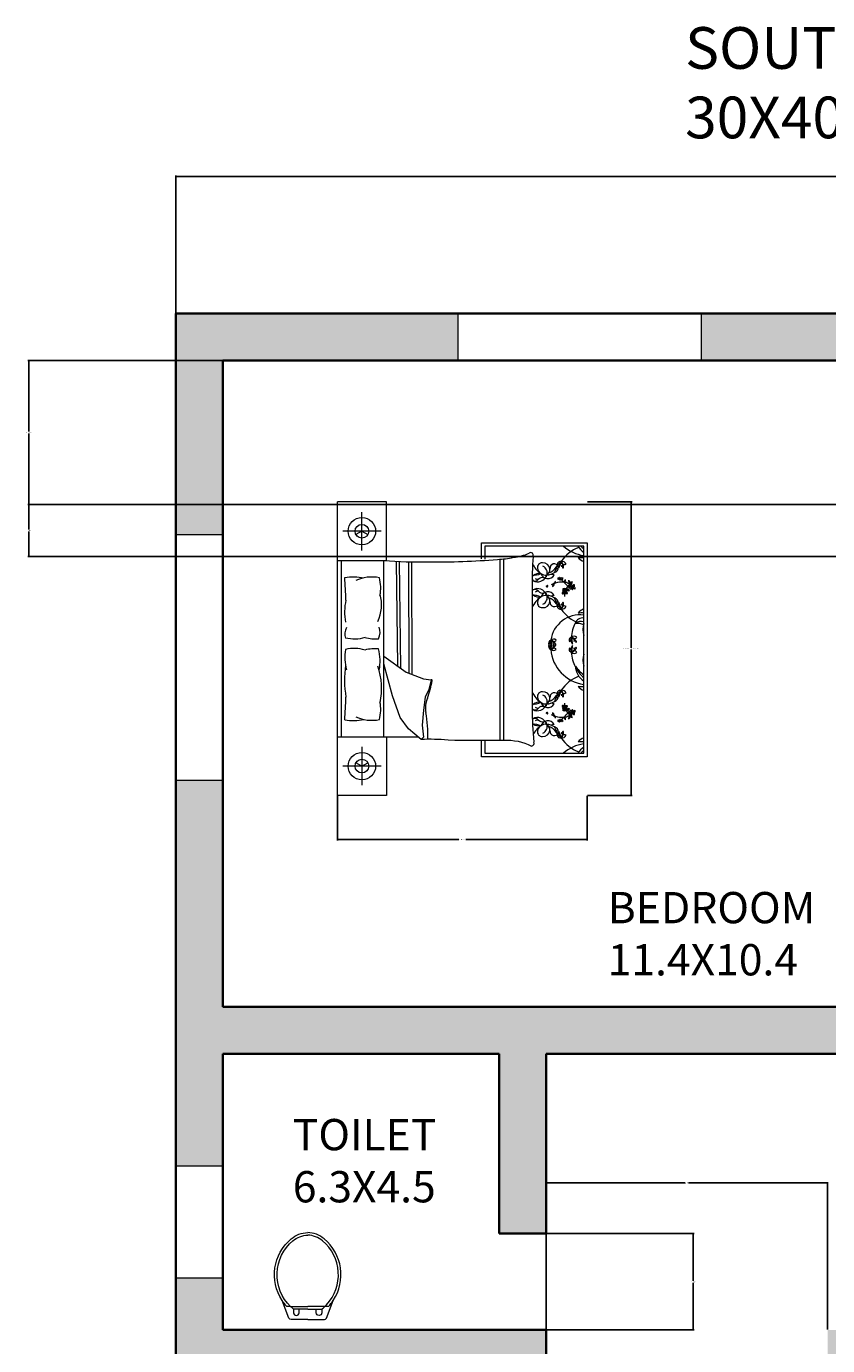
# Model space of a CAD drawing. Units: inches. Extents: x 8 to 486, y -516 to 97.
# Tile 3 of 5: x 8 to 162, y -185 to 68. Entities that reach past the tile are written whole.
import ezdxf

# ---------------------------------------------------------------- set-up
doc = ezdxf.new("R2010")
doc.units = ezdxf.units.IN
doc.header["$MEASUREMENT"] = 0
for name, color, linetype, lineweight in [('A-ANNO-DIMS', 2, 'Continuous', 18), ('A-ANNO-TEXT', 7, 'Continuous', 25), ('A-AREA-IDEN', 7, 'Continuous', 18), ('A-FLOR-FIXT', 9, 'Continuous', 18), ('A-FURN', 8, 'Continuous', 18), ('A-GLAZ', 4, 'Continuous', 18), ('A-WALL', 7, 'Continuous', 35), ('A-WALL-PATT', 150, 'Continuous', 13)]:
    doc.layers.add(name, color=color, linetype=linetype, lineweight=lineweight)
doc.styles.get("Standard").update_dxf_attribs({"font": 'arial.ttf'})
doc.dimstyles.get("Standard").update_dxf_attribs({"dimtxt": 0.18, "dimasz": 0.18, "dimexe": 0.18, "dimexo": 0.0625, "dimgap": 0.09, "dimtad": 0, "dimtih": 1, "dimtoh": 1, "dimdec": 0, "dimzin": 0, "dimdsep": 46, "dimlunit": 3, "dimtxsty": 'Standard', "dimcen": 0.09, "dimadec": 0, "dimazin": 0, "dimtfac": 1, "dimtdec": 0, "dimtofl": 0, "dimtmove": 0, "dimatfit": 3, "dimfxl": 1, "dimtolj": 1, "dimtzin": 0, "dimarcsym": 0})

# ---------------------------------------------------------------- blocks, each defined once
blk = doc.blocks.new('*D1')
at = {"layer": 'A-ANNO-DIMS', "color": 0, "lineweight": -2, "transparency": 16777216}
for p, q in [((37.13, 12.8), (37.13, 39.25)), ((37.31, 39.07), (214.23, 39.07)), ((411.95, 39.07), (235.02, 39.07)), ((412.13, 12.8), (412.13, 39.25))]:
    blk.add_line(p, q, dxfattribs=at)
at = {"layer": 'A-ANNO-DIMS', "color": 0, "transparency": 16777216}
for points in [[(37.31, 39.1), (37.31, 39.04), (37.13, 39.07)], [(411.95, 39.1), (411.95, 39.04), (412.13, 39.07)]]:
    blk.add_solid(points, dxfattribs=at)
at = {"layer": 'Defpoints', "color": 0, "transparency": 16777216}
for p in [(412.13, 39.07), (37.13, 12.74), (412.13, 12.74)]:
    blk.add_point(p, dxfattribs=at)
at = {"layer": 'A-ANNO-DIMS', "color": 0, "transparency": 16777216, "insert": (224.63, 39.07), "char_height": 6, "attachment_point": 5}
blk.add_mtext('\\A1;31\'-3"', dxfattribs=at)
blk = doc.blocks.new('BED-DOUBLE')
for p, q in [((0, 0), (0, 56.34)), ((4.7, 47.03), (4.7, 54.39)), ((8.38, 50.71), (1.01, 50.71)), ((27.62, 45.39), (27.62, 48.51)), ((27.62, 48.51), (47.92, 48.51)), ((47.92, 48.51), (47.92, 7.44)), ((28.27, 47.86), (28.27, 45.37)), ((47.26, 47.86), (28.27, 47.86)), ((47.26, 8.09), (47.26, 47.86)), ((0.72, 45.07), (0.72, 11.27)), ((8.9, 11.27), (8.9, 45.07)), ((11.24, 44.92), (11.53, 24.86)), ((11.82, 44.9), (12.11, 24.44)), ((13.6, 44.87), (13.68, 23.48)), ((14.18, 44.87), (14.26, 23.26)), ((31.13, 45.33), (31.13, 10.62)), ((31.84, 45.38), (31.84, 10.62)), ((41.55, 42.31), (40.91, 42.43)), ((37.37, 39.61), (37.37, 16.73)), ((41.55, 38.37), (40.91, 38.24)), ((8.9, 26.75), (13.2, 23.66)), ((10.58, 19.09), (8.9, 25.24)), ((13.2, 23.66), (16.51, 22.4)), ((16.51, 22.4), (17.99, 22.17)), ((17.54, 20.35), (16.85, 18.87)), ((17.99, 22.17), (17.54, 20.35)), ((12.06, 14.99), (10.58, 19.09)), ((16.85, 18.87), (16.51, 16.36)), ((16.51, 16.36), (16.28, 13.5)), ((41.55, 17.58), (40.91, 17.7)), ((13.66, 12.82), (12.06, 14.99)), ((16.05, 10.76), (13.66, 12.82)), ((16.28, 13.5), (16.51, 11.22)), ((41.55, 13.64), (40.91, 13.52)), ((0, 11.27), (15.46, 11.27)), ((16.51, 11.22), (16.05, 10.76)), ((27.62, 7.44), (27.62, 10.62)), ((28.27, 10.62), (28.27, 8.09)), ((4.7, 9.31), (4.7, 1.95)), ((28.27, 8.09), (47.26, 8.09)), ((8.38, 5.63), (1.01, 5.63)), ((47.92, 7.44), (27.62, 7.44))]:
    blk.add_line(p, q)
for points in [[(0, 45.07), (9.39, 45.07), (9.39, 56.34), (0, 56.34)], [(4.7, 50.71), (3.56, 50.05)], [(4.7, 50.71), (5.83, 50.05)], [(9.39, 11.27), (9.39, 0), (0, 0)], [(4.7, 5.63), (3.56, 6.29)], [(4.7, 5.63), (5.83, 6.29)]]:
    blk.add_lwpolyline(points)
for points in [[(30.69, 45.31, 0.056112), (33.79, 45.72, 0.095341), (36.78, 46.51)], [(1.4, 41.84, -0.074897), (5.08, 41.77, 0.472817)], [(5.29, 30.31, -0.14099), (1.54, 30.2, -0.235245)], [(5.29, 27.91, 0.14099), (1.54, 28.02, 0.235245)], [(1.4, 14.5, 0.074897), (5.08, 14.57, -0.472817)], [(21.21, 10.65, 0.001242), (31.9, 10.62, -0.127202), (37.23, 9.49)]]:
    blk.add_lwpolyline(points, format="xyb")
for centre, radius in [((4.7, 50.71), 2.63), ((4.7, 50.71), 1.31), ((43.59, 39.05), 0.143), ((45.1, 39.99), 0.143), ((43.59, 16.9), 0.143), ((45.1, 15.96), 0.143), ((4.7, 5.63), 2.63), ((4.7, 5.63), 1.31)]:
    blk.add_circle(centre, radius)
for centre, radius, start, end in [((37.06, 46.09), 0.514, 336.5219, 123.8264), ((92.17, 41.33), 54.82, 175.2402, 181.8035), ((48.98, 40.75), 7.36, 111.4092, 145.6135), ((48.25, 53.34), 7.36, 228.1144, 262.255), ((49.24, 49.64), 3.59, 209.8884, 236.5383), ((48.41, 47.64), 2.99, 221.0454, 247.4453), ((46.8, 55.83), 10.18, 266.3481, 272.5919), ((49.91, 50.93), 4.47, 223.5186, 233.6964), ((15.79, 146.07), 101.24, 266.1, 270.9282), ((19.47, 176.89), 132.06, 269.1145, 274.8735), ((41.34, 46.16), 4.26, 203.6453, 236.3329), ((39.29, 43.68), 0.951, 88.9462, 185.5144), ((39.99, 43.97), 1.69, 193.079, 274.7067), ((39.43, 43.29), 1.35, 7.1143, 95.0551), ((38.92, 42.76), 1.31, 338.5779, 68.4181), ((39.13, 43.52), 1.64, 305.9599, 357.6409), ((39.73, 45.27), 2.66, 288.2955, 328.7386), ((41.6, 43.6), 0.846, 19.1312, 189.736), ((41.34, 43.8), 1.06, 285.6955, 4.031), ((42.75, 42.66), 1.12, 128.4175, 173.8338), ((42.51, 43.77), 0.518, 126.7319, 206.0245), ((42.76, 44.31), 0.61, 76.272, 177.0484), ((41.84, 45.56), 1.26, 284.7031, 328.6173), ((43.59, 43.96), 1.16, 125.7657, 194.5347), ((37.88, 46.02), 5.15, 332.8176, 347.4827), ((43.08, 44.11), 0.816, 20.9613, 102.2885), ((43.52, 44.92), 0.614, 181.7131, 301.5367), ((41.51, 43.68), 1.86, 2.0648, 41.1598), ((42.63, 44.37), 0.602, 316.2238, 62.3173), ((42.98, 44.02), 0.048, 20.2667, 316.2271), ((43.23, 43.75), 0.0444, 52.0591, 168.5166), ((43.28, 43.74), 0.0914, 168.5166, 2.0648), ((-534.78, 10.78), 537.08, 2.8502, 3.3148), ((6.56, 34.66), 7.26, 78.2417, 114.8684), ((0.75, 39.83), 7.55, 348.9631, 14.8961), ((37.99, 41.7), 0.679, 196.6343, 225.5483), ((37.79, 44.6), 2.33, 259.249, 301.1782), ((37.99, 41.7), 0.679, 127.675, 162.5814), ((38.39, 42.79), 1.8, 240.8249, 340.7178), ((37.86, 41.99), 0.843, 246.1646, 318.4347), ((38.8, 40.44), 2.17, 85.2696, 124.215), ((38.72, 43.06), 1.62, 240.0851, 262.564), ((39.35, 40.67), 1.16, 74.8529, 138.4347), ((40.34, 43), 1.4, 196.8663, 330.0915), ((39.75, 42.12), 0.35, 254.8529, 12.6959), ((38.8, 40.44), 2.17, 53.6555, 57.2989), ((39.95, 45.3), 3.02, 273.4924, 303.7117), ((43.11, 36.27), 4.67, 110.1059, 116.9968), ((41.52, 40.48), 0.115, 83.9457, 185.6216), ((41.06, 40.58), 0.472, 328.836, 0.8141), ((41.3, 40.45), 0.27, 306.5232, 32.4668), ((41.62, 40.66), 0.115, 112.5583, 214.2343), ((41.55, 40.86), 0.27, 265.7131, 351.6568), ((41.31, 41.01), 0.472, 297.3659, 329.344), ((40.95, 41.42), 0.905, 313.6929, 321.7899), ((41.96, 40.8), 0.296, 115.5379, 168.6744), ((40.95, 41.22), 0.89, 329.344, 349.7412), ((43.11, 36.27), 4.67, 86.1723, 106.4158), ((40.24, 41.02), 1.59, 352.8698, 1.6736), ((42.35, 41.59), 0.111, 125.0752, 284.7644), ((42.52, 41.63), 0.239, 127.3642, 168.4363), ((42.33, 41.83), 0.345, 277.4968, 341.2737), ((42.6, 41.67), 0.137, 88.1325, 178.8919), ((42.88, 41.52), 0.297, 136.3462, 189.6513), ((42.71, 41.49), 0.124, 189.6513, 312.3208), ((42.74, 41.83), 0.143, 183.2768, 356.7232), ((43.19, 41.58), 0.47, 164.2829, 186.9148), ((42.63, 41.57), 0.235, 312.3208, 40.2111), ((43.13, 41.84), 0.333, 201.6382, 274.947), ((42.69, 41.38), 0.436, 42.3896, 66.5724), ((47.08, 44.83), 5.35, 217.9541, 226.8459), ((43, 41.64), 0.237, 10.9597, 52.2379), ((43.15, 41.62), 0.11, 274.947, 37.5263), ((43.52, 40.99), 0.115, 112.5583, 214.2343), ((43.45, 41.2), 0.27, 265.7131, 351.6568), ((43.21, 41.35), 0.472, 297.3659, 329.344), ((43.23, 38.6), 2.34, 60.7959, 85.244), ((38.25, 35.23), 7.7, 37.8256, 47.7588), ((42.85, 41.75), 0.905, 313.6929, 321.7899), ((43.85, 41.13), 0.296, 115.5379, 168.6744), ((42.85, 41.56), 0.89, 329.344, 349.7412), ((42.14, 41.35), 1.59, 352.8698, 1.6736), ((44.37, 41.03), 0.16, 33.0979, 123.1364), ((40.84, 38.77), 4.19, 31.1156, 34.8118), ((44.14, 40.76), 0.434, 2.3172, 70.5201), ((43.93, 40.29), 0.654, 310.9365, 22.7695), ((44.5, 40.65), 0.125, 135.7354, 318.1297), ((44.29, 40.86), 0.166, 315.7354, 31.1156), ((44.15, 40.5), 0.385, 319.3812, 5.5456), ((44.59, 40.65), 0.125, 68.2452, 250.6395), ((44.3, 40.81), 0.374, 352.6008, 57.1845), ((45.64, 38.3), 2.5, 111.7087, 116.2181), ((43.23, 38.6), 2.34, 47.5083, 55.9967), ((44.66, 40.89), 0.374, 252.8042, 349.6943), ((44.3, 40.22), 0.398, 331.1838, 51.6792), ((44.7, 40.92), 0.166, 248.2452, 323.6254), ((44.55, 41.02), 0.434, 291.7087, 3.0299), ((41.46, 43.31), 4.19, 323.6254, 327.3216), ((44.89, 40.92), 0.16, 325.6077, 55.6462), ((1.3, 36.57), 7.17, 333.8761, 16.1746), ((37.99, 38.97), 0.679, 134.4517, 156.7144), ((37.99, 38.97), 0.679, 203.2856, 232.325), ((37.79, 36.08), 2.33, 58.8218, 100.2867), ((41.34, 34.52), 4.26, 123.6671, 158.5059), ((38.39, 37.89), 1.8, 19.2822, 119.1751), ((37.86, 38.68), 0.843, 41.5653, 113.8354), ((38.8, 40.23), 2.17, 235.785, 274.7304), ((38.72, 37.62), 1.62, 97.436, 119.9149), ((39.99, 36.71), 1.69, 85.2933, 166.921), ((39.35, 40.01), 1.16, 221.5653, 285.1471), ((40.34, 37.67), 1.4, 29.9085, 163.1337), ((38.92, 37.92), 1.31, 291.5819, 21.4221), ((39.75, 38.56), 0.35, 347.3041, 105.1471), ((38.8, 40.23), 2.17, 302.7011, 306.3445), ((40.21, 40.19), 0.177, 169.5864, 349.5616), ((39.13, 37.16), 1.64, 2.3591, 54.0401), ((39.95, 35.38), 3.02, 56.2883, 86.5076), ((40.28, 40.18), 0.109, 349.5616, 167.2949), ((41.55, 40.12), 0.296, 129.5056, 182.6421), ((40.7, 40.8), 0.89, 308.4388, 328.836), ((40.54, 41.53), 1.59, 296.5064, 305.3102), ((40.53, 40.71), 0.905, 336.3901, 344.4871), ((43.2, 38.81), 0.111, 125.0752, 284.7644), ((43.37, 38.85), 0.239, 93.635, 168.4363), ((43.38, 40.15), 0.654, 253.6301, 325.4631), ((43.56, 39.24), 0.463, 82.0748, 142.6895), ((43.51, 39.88), 0.475, 228.342, 274.9894), ((43.34, 39.23), 0.141, 138.2946, 276.2474), ((43.39, 39.21), 0.196, 358.5719, 143.8954), ((43.18, 39.05), 0.345, 277.4968, 341.2737), ((43.46, 38.88), 0.137, 88.1325, 178.8919), ((43.51, 39.36), 0.197, 208.8493, 269.9355), ((43.34, 39.32), 0.226, 274.2123, 318.1587), ((43.73, 38.74), 0.297, 136.3462, 189.6513), ((43.56, 38.71), 0.124, 189.6513, 312.3208), ((46.34, 38.35), 2.81, 175.2415, 182.8929), ((43.52, 39.8), 0.398, 273.8774, 357.1501), ((44.04, 38.79), 0.47, 164.2829, 186.9148), ((44.03, 39.09), 0.452, 121.9501, 165.2442), ((43.68, 40.08), 0.385, 262.0748, 308.2393), ((43.49, 38.79), 0.235, 312.3208, 40.2111), ((43.98, 39.06), 0.333, 201.6382, 274.947), ((43.71, 39.26), 0.095, 262.868, 7.094), ((43.54, 38.6), 0.436, 42.3896, 66.5724), ((43.7, 39.34), 0.283, 278.5614, 22.5914), ((43.86, 38.86), 0.237, 10.9597, 118.7804), ((46.34, 38.35), 2.81, 156.1523, 156.9499), ((43.86, 39.35), 0.142, 44.3732, 121.9501), ((44.3, 39.69), 0.398, 181.4625, 249.4747), ((46.34, 38.35), 2.81, 130.182, 149.456), ((44.23, 40), 0.385, 215.1128, 261.2773), ((44.54, 39.98), 0.654, 197.889, 269.722), ((44, 38.83), 0.11, 274.947, 37.5263), ((44.34, 39.76), 0.475, 248.3627, 295.0101), ((44.1, 39.16), 0.463, 20.6625, 81.2773), ((44.79, 39.95), 0.463, 139.3812, 199.9959), ((44.23, 40.25), 0.475, 285.6484, 332.2957), ((44.71, 39.75), 0.111, 125.0752, 284.7644), ((44.88, 39.79), 0.239, 93.635, 168.4363), ((44.85, 40.17), 0.141, 138.2946, 276.2474), ((44.69, 39.98), 0.345, 277.4968, 341.2737), ((44.9, 40.15), 0.196, 358.5719, 143.8954), ((44.97, 39.82), 0.137, 88.1325, 178.8919), ((45.02, 40.3), 0.197, 208.8493, 269.9355), ((44.85, 40.26), 0.226, 274.2123, 318.1587), ((45.24, 39.68), 0.297, 136.3462, 189.6513), ((45.07, 39.65), 0.124, 189.6513, 312.3208), ((45.55, 39.73), 0.47, 164.2829, 186.9148), ((45.54, 40.03), 0.452, 121.9501, 165.2442), ((45, 39.73), 0.235, 312.3208, 40.2111), ((45.5, 39.99), 0.333, 201.6382, 274.947), ((45.23, 40.2), 0.095, 262.868, 7.094), ((45.05, 39.54), 0.436, 42.3896, 66.5724), ((45.21, 40.28), 0.283, 278.5614, 22.5914), ((45.37, 39.79), 0.237, 10.9597, 118.7804), ((45.37, 40.29), 0.142, 44.3732, 121.9501), ((45.52, 39.77), 0.11, 274.947, 37.5263), ((11.26, 35.15), 9.9, 166.3427, 191.1841), ((39.29, 37), 0.951, 174.4856, 271.0538), ((39.43, 37.39), 1.35, 264.9449, 352.8857), ((39.73, 35.4), 2.66, 31.2614, 71.7045), ((41.6, 37.08), 0.846, 170.264, 340.8688), ((42.75, 38.01), 1.12, 186.1662, 231.5825), ((41.34, 36.88), 1.06, 355.969, 74.3045), ((42.51, 36.91), 0.518, 153.9755, 233.2681), ((42.76, 36.36), 0.61, 182.9516, 283.728), ((41.84, 35.12), 1.26, 31.3827, 75.2969), ((43.59, 36.72), 1.16, 165.4653, 234.2343), ((37.88, 34.66), 5.15, 12.5173, 27.1824), ((41.51, 37), 1.86, 318.8402, 357.9352), ((42.63, 36.3), 0.602, 297.6827, 43.7762), ((43.52, 35.75), 0.614, 58.4633, 178.2869), ((43.08, 36.57), 0.816, 257.7115, 339.0387), ((48.98, 39.93), 7.36, 214.3865, 248.5908), ((43.01, 36.67), 0.0796, 43.7762, 339.7183), ((43.28, 36.93), 0.0914, 357.9352, 191.4834), ((43.23, 36.92), 0.0444, 191.4834, 307.9409), ((48.41, 33.04), 2.99, 112.5547, 138.9546), ((46.55, 28.98), 5.69, 82.8636, 171.8197), ((52.19, 29.78), 7.36, 152.5854, 175.5377), ((46.95, 32.74), 1.32, 76.3898, 169.0739), ((46.77, 31.74), 1.67, 72.8609, 131.9049), ((46.03, 29.72), 3.29, 68.117, 96.6195), ((46.8, 24.84), 10.18, 87.4081, 93.6519), ((51.13, 31.84), 4.05, 162.9798, 196.4569), ((4.21, 30.97), 2.79, 153.3437, 196.1026), ((5.19, 31.35), 2.99, 335.0183, 18.5407), ((45.41, 29.75), 0.816, 50.8855, 132.2127), ((45.38, 30.68), 0.614, 211.6373, 331.4609), ((53.22, 30.24), 5.98, 174.3643, 175.6213), ((57.31, 27.08), 10.69, 160.0972, 160.2783), ((11.47, 26.54), 10.04, 171.5249, 193.96), ((7.17, 36.95), 6.9, 254.1707, 275.9871), ((7.17, 21.26), 6.9, 84.0129, 105.8293), ((-1.76, 25.79), 9.94, 349.8617, 13.6238), ((41.09, 29.2), 0.61, 106.1963, 206.9726), ((41.09, 28.62), 0.61, 153.0274, 253.8037), ((39.66, 29.82), 1.26, 314.6273, 358.5415), ((39.66, 28), 1.26, 1.4585, 45.3727), ((41.98, 29.31), 1.16, 155.6899, 224.4589), ((41.98, 28.51), 1.16, 135.5411, 204.3101), ((41.47, 29.19), 0.816, 50.8855, 132.2127), ((41.44, 30.11), 0.614, 211.6373, 331.4609), ((40.94, 29.19), 0.602, 346.148, 92.2415), ((40.32, 28.03), 1.86, 31.989, 71.0841), ((36.01, 28.25), 5.15, 2.7418, 17.407), ((36.01, 29.58), 5.15, 342.593, 357.2582), ((40.32, 29.8), 1.86, 288.9159, 328.011), ((40.94, 28.64), 0.602, 267.7585, 13.852), ((41.44, 27.71), 0.614, 28.5391, 148.3627), ((41.47, 28.64), 0.816, 227.7873, 309.1145), ((48.25, 28.61), 7.36, 184.4623, 262.255), ((41.42, 29.06), 0.048, 50.1909, 346.0209), ((41.45, 28.76), 0.0796, 13.852, 309.9245), ((41.82, 28.97), 0.0914, 198.4408, 31.989), ((41.77, 28.95), 0.0444, 81.9833, 198.4408), ((41.82, 28.86), 0.0914, 328.011, 161.5592), ((41.77, 28.87), 0.0444, 161.5592, 278.0167), ((45.03, 29.77), 0.61, 106.1963, 206.9726), ((45.03, 28.06), 0.61, 153.0274, 253.8037), ((43.6, 30.38), 1.26, 314.6273, 358.5415), ((43.6, 27.44), 1.26, 1.4585, 45.3727), ((45.92, 29.87), 1.16, 155.6899, 224.4589), ((45.92, 27.95), 1.16, 135.5411, 204.3101), ((44.26, 28.59), 1.86, 31.989, 71.0841), ((39.95, 28.81), 5.15, 2.7418, 17.407), ((44.88, 29.75), 0.602, 346.148, 92.2415), ((39.95, 29.01), 5.15, 342.593, 357.2582), ((44.26, 29.23), 1.86, 288.9159, 328.011), ((44.88, 28.07), 0.602, 267.7585, 13.852), ((45.36, 29.62), 0.048, 50.1909, 346.0209), ((45.39, 28.2), 0.0796, 13.852, 309.9245), ((45.76, 29.53), 0.0914, 198.4408, 31.989), ((45.71, 29.52), 0.0444, 81.9833, 198.4408), ((45.76, 28.3), 0.0914, 328.011, 161.5592), ((45.71, 28.31), 0.0444, 161.5592, 278.0167), ((45.38, 27.15), 0.614, 28.5391, 148.3627), ((45.41, 28.08), 0.816, 227.7873, 309.1145), ((52.19, 28.04), 7.36, 184.4623, 207.4146), ((51.13, 25.99), 4.05, 163.5431, 197.0202), ((53.22, 27.59), 5.98, 184.3787, 185.6357), ((57.31, 30.74), 10.69, 199.7217, 199.9028), ((21.79, 22.22), 20.43, 172.2196, 189.497), ((-4.62, 20.49), 13.1, 348.0397, 19.2615), ((48.98, 16.02), 7.36, 111.4092, 145.6135), ((49.24, 24.92), 3.59, 181.272, 236.5383), ((51.16, 28.56), 6.65, 214.0123, 234.053), ((49.91, 26.21), 4.47, 197.8504, 233.6964), ((-3.3, 26.09), 21.85, 340.1194, 349.3383), ((18.04, 22.05), 0.136, 358.8623, 109.7536), ((46.8, 31.1), 10.18, 266.3481, 272.5919), ((48.41, 22.91), 2.99, 221.0454, 247.4453), ((-534.78, 45.56), 537.08, 356.6852, 357.1498), ((0.75, 16.51), 7.55, 345.1039, 11.0369), ((21.45, 16.81), 4.59, 156.2616, 191.3392), ((41.34, 21.43), 4.26, 201.4941, 236.3329), ((37.79, 19.87), 2.33, 259.7133, 301.1782), ((38.8, 15.72), 2.17, 85.2696, 124.215), ((39.29, 18.95), 0.951, 88.9462, 185.5144), ((39.99, 19.24), 1.69, 193.079, 274.7067), ((40.34, 18.28), 1.4, 196.8663, 330.0915), ((39.43, 18.56), 1.35, 7.1143, 95.0551), ((38.92, 18.03), 1.31, 338.5779, 68.4181), ((39.13, 18.79), 1.64, 305.9599, 357.6409), ((39.95, 20.57), 3.02, 273.4924, 303.7117), ((39.73, 20.54), 2.66, 288.2955, 328.7386), ((41.6, 18.87), 0.846, 19.1312, 189.736), ((41.34, 19.07), 1.06, 285.6955, 4.031), ((42.75, 17.93), 1.12, 128.4175, 173.8338), ((42.51, 19.04), 0.518, 126.7319, 206.0245), ((42.76, 19.58), 0.61, 76.272, 177.0484), ((41.84, 20.83), 1.26, 284.7031, 328.6173), ((43.59, 19.23), 1.16, 125.7657, 194.5347), ((37.88, 21.29), 5.15, 332.8176, 347.4827), ((43.08, 19.38), 0.816, 20.9613, 102.2885), ((42.63, 19.64), 0.602, 316.2238, 62.3173), ((41.51, 18.95), 1.86, 2.0648, 41.1598), ((43.52, 20.19), 0.614, 181.7131, 301.5367), ((42.98, 19.29), 0.048, 20.2667, 316.2271), ((43.23, 19.02), 0.0444, 52.0591, 168.5166), ((43.28, 19.02), 0.0914, 168.5166, 2.0648), ((46.34, 17.59), 2.81, 177.1071, 184.7585), ((-3.9, 11.73), 21.26, 357.4519, 11.3392), ((37.99, 16.98), 0.679, 127.675, 156.7144), ((96.02, 16.06), 58.65, 179.3433, 185.6887), ((37.99, 16.98), 0.679, 203.229, 225.5483), ((38.39, 18.06), 1.8, 240.8249, 340.7178), ((37.86, 17.26), 0.843, 246.1646, 318.4347), ((38.72, 18.33), 1.62, 240.0851, 262.564), ((39.35, 15.94), 1.16, 74.8529, 138.4347), ((39.75, 17.39), 0.35, 254.8529, 12.6959), ((38.8, 15.72), 2.17, 53.6555, 57.2989), ((40.21, 15.76), 0.177, 10.4384, 190.4136), ((40.28, 15.77), 0.109, 192.7051, 10.4384), ((43.11, 19.68), 4.67, 243.0032, 249.8941), ((40.7, 15.15), 0.89, 31.164, 51.5612), ((41.55, 15.83), 0.296, 177.3579, 230.4944), ((40.54, 14.42), 1.59, 54.6898, 63.4936), ((40.53, 15.24), 0.905, 15.5129, 23.6099), ((41.52, 15.47), 0.115, 174.3784, 276.0543), ((41.3, 15.5), 0.27, 327.5332, 53.4768), ((41.06, 15.36), 0.472, 359.1859, 31.164), ((41.62, 15.29), 0.115, 145.7657, 247.4417), ((41.55, 15.09), 0.27, 8.3432, 94.2869), ((41.31, 14.94), 0.472, 30.656, 62.6341), ((43.11, 19.68), 4.67, 253.5842, 273.8277), ((43.2, 17.14), 0.111, 75.2356, 234.9248), ((43.37, 17.09), 0.239, 191.5637, 266.365), ((43.51, 16.07), 0.475, 85.0106, 131.658), ((43.38, 15.8), 0.654, 34.5369, 106.3699), ((43.56, 16.71), 0.463, 217.3105, 277.9252), ((43.34, 16.72), 0.141, 83.7526, 221.7054), ((43.18, 16.9), 0.345, 18.7263, 82.5032), ((43.39, 16.74), 0.196, 216.1046, 1.4281), ((43.46, 17.06), 0.137, 181.1081, 271.8675), ((43.51, 16.58), 0.197, 90.0645, 151.1507), ((43.34, 16.63), 0.226, 41.8413, 85.7877), ((38.25, 20.72), 7.7, 312.2412, 322.1744), ((43.23, 17.35), 2.34, 274.756, 299.2041), ((43.73, 17.21), 0.297, 170.3487, 223.6538), ((43.56, 17.24), 0.124, 47.6792, 170.3487), ((43.52, 16.15), 0.398, 2.8499, 86.1226), ((44.04, 17.15), 0.47, 173.0852, 195.7171), ((44.03, 16.86), 0.452, 194.7558, 238.0499), ((43.68, 15.87), 0.385, 51.7607, 97.9252), ((43.49, 17.16), 0.235, 319.7889, 47.6792), ((43.98, 16.89), 0.333, 85.053, 158.3618), ((43.71, 16.68), 0.095, 352.906, 97.132), ((43.54, 17.35), 0.436, 293.4276, 317.6104), ((43.86, 17.09), 0.237, 241.2196, 349.0403), ((43.7, 16.6), 0.283, 337.4086, 81.4386), ((46.34, 17.59), 2.81, 203.0501, 203.8477), ((43.86, 16.59), 0.142, 238.0499, 315.6268), ((44.3, 16.26), 0.398, 110.5253, 178.5375), ((44.54, 15.97), 0.654, 90.278, 162.111), ((44.23, 15.95), 0.385, 98.7227, 144.8872), ((46.34, 17.59), 2.81, 210.544, 229.818), ((44, 17.11), 0.11, 322.4737, 85.053), ((44.34, 16.19), 0.475, 64.9899, 111.6373), ((44.1, 16.78), 0.463, 278.7227, 339.3375), ((44.79, 15.99), 0.463, 160.0041, 220.6188), ((43.93, 15.66), 0.654, 337.2305, 49.0635), ((44.23, 15.7), 0.475, 27.7043, 74.3516), ((44.5, 15.3), 0.125, 41.8703, 224.2646), ((44.29, 15.09), 0.166, 328.8844, 44.2646), ((44.15, 15.44), 0.385, 354.4544, 40.6188), ((44.59, 15.29), 0.125, 109.3605, 291.7548), ((44.3, 15.14), 0.374, 302.8155, 7.3992), ((45.64, 17.65), 2.5, 243.7819, 248.2913), ((43.23, 17.35), 2.34, 304.0033, 312.4917), ((44.3, 15.72), 0.398, 308.3208, 28.8162), ((44.66, 15.06), 0.374, 10.3057, 107.1958), ((44.71, 16.2), 0.111, 75.2356, 234.9248), ((44.7, 15.02), 0.166, 36.3746, 111.7548), ((44.88, 16.16), 0.239, 191.5637, 266.365), ((44.85, 15.78), 0.141, 83.7526, 221.7054), ((44.55, 14.92), 0.434, 356.9701, 68.2913), ((44.69, 15.96), 0.345, 18.7263, 82.5032), ((44.9, 15.8), 0.196, 216.1046, 1.4281), ((44.97, 16.12), 0.137, 181.1081, 271.8675), ((45.02, 15.65), 0.197, 90.0645, 151.1507), ((44.85, 15.69), 0.226, 41.8413, 85.7877), ((45.07, 16.3), 0.124, 47.6792, 170.3487), ((45.24, 16.27), 0.297, 170.3487, 223.6538), ((45.55, 16.21), 0.47, 173.0852, 195.7171), ((45.54, 15.92), 0.452, 194.7558, 238.0499), ((45, 16.22), 0.235, 319.7889, 47.6792), ((45.5, 15.95), 0.333, 85.053, 158.3618), ((45.23, 15.75), 0.095, 352.906, 97.132), ((45.05, 16.41), 0.436, 293.4276, 317.6104), ((45.37, 16.15), 0.237, 241.2196, 349.0403), ((45.21, 15.67), 0.283, 337.4086, 81.4386), ((45.37, 15.66), 0.142, 238.0499, 315.6268), ((45.52, 16.18), 0.11, 322.4737, 85.053), ((6.56, 21.68), 7.26, 245.1316, 281.7583), ((37.99, 14.24), 0.679, 134.4517, 153.558), ((37.99, 14.24), 0.679, 210.0293, 232.325), ((37.79, 11.35), 2.33, 58.8218, 99.1554), ((38.39, 13.16), 1.8, 19.2822, 119.1751), ((37.86, 13.96), 0.843, 41.5653, 113.8354), ((41.34, 9.79), 4.26, 123.6671, 153.2997), ((38.8, 15.5), 2.17, 235.785, 274.7304), ((38.72, 12.89), 1.62, 97.436, 119.9149), ((39.99, 11.98), 1.69, 85.2933, 166.921), ((39.35, 15.28), 1.16, 221.5653, 285.1471), ((40.34, 12.94), 1.4, 29.9085, 163.1337), ((38.92, 13.19), 1.31, 291.5819, 21.4221), ((39.75, 13.83), 0.35, 347.3041, 105.1471), ((38.8, 15.5), 2.17, 302.7011, 306.3445), ((39.13, 12.43), 1.64, 2.3591, 54.0401), ((39.95, 10.65), 3.02, 56.2883, 86.5076), ((39.73, 10.68), 2.66, 31.2614, 71.7045), ((40.95, 14.53), 0.905, 38.2101, 46.3071), ((41.34, 12.15), 1.06, 355.969, 74.3045), ((42.75, 13.29), 1.12, 186.1662, 231.5825), ((41.96, 15.15), 0.296, 191.3256, 244.4621), ((40.95, 14.72), 0.89, 10.2588, 30.656), ((40.24, 14.93), 1.59, 358.3264, 7.1302), ((42.35, 14.36), 0.111, 75.2356, 234.9248), ((42.52, 14.31), 0.239, 191.5637, 232.6358), ((42.33, 14.12), 0.345, 18.7263, 82.5032), ((42.6, 14.28), 0.137, 181.1081, 271.8675), ((42.88, 14.43), 0.297, 170.3487, 223.6538), ((42.71, 14.46), 0.124, 47.6792, 170.3487), ((42.74, 14.11), 0.143, 3.2768, 176.7232), ((43.19, 14.37), 0.47, 173.0852, 195.7171), ((42.63, 14.37), 0.235, 319.7889, 47.6792), ((43.13, 14.11), 0.333, 85.053, 158.3618), ((42.69, 14.57), 0.436, 293.4276, 317.6104), ((47.08, 11.12), 5.35, 133.1541, 142.0459), ((43, 14.31), 0.237, 307.7621, 349.0403), ((43.15, 14.33), 0.11, 322.4737, 85.053), ((43.52, 14.96), 0.115, 145.7657, 247.4417), ((43.45, 14.75), 0.27, 8.3432, 94.2869), ((43.21, 14.6), 0.472, 30.656, 62.6341), ((42.85, 14.2), 0.905, 38.2101, 46.3071), ((43.85, 14.81), 0.296, 191.3256, 244.4621), ((42.85, 14.39), 0.89, 10.2588, 30.656), ((42.14, 14.59), 1.59, 358.3264, 7.1302), ((44.14, 15.19), 0.434, 289.4799, 357.6828), ((40.84, 17.17), 4.19, 325.1882, 328.8844), ((44.37, 14.91), 0.16, 236.8636, 326.9021), ((41.46, 12.64), 4.19, 32.6784, 36.3746), ((44.89, 15.03), 0.16, 304.3538, 34.3923), ((17.45, -40.9), 51.68, 85.8294, 91.553), ((37.19, 10.01), 0.52, 273.98, 27.3412), ((39.29, 12.27), 0.951, 174.4856, 271.0538), ((39.43, 12.66), 1.35, 264.9449, 352.8857), ((41.6, 12.35), 0.846, 170.264, 340.8688), ((42.51, 12.18), 0.518, 153.9755, 233.2681), ((41.84, 10.39), 1.26, 31.3827, 75.2969), ((42.76, 11.64), 0.61, 182.9516, 283.728), ((43.59, 11.99), 1.16, 165.4653, 234.2343), ((37.88, 9.93), 5.15, 12.5173, 27.1824), ((41.51, 12.27), 1.86, 318.8402, 357.9352), ((42.63, 11.58), 0.602, 297.6827, 43.7762), ((43.52, 11.03), 0.614, 58.4633, 178.2869), ((43.08, 11.84), 0.816, 257.7115, 339.0387), ((48.98, 15.2), 7.36, 214.3865, 248.5908), ((43.01, 11.94), 0.0796, 43.7762, 339.7183), ((43.28, 12.2), 0.0914, 357.9352, 191.4834), ((43.23, 12.2), 0.0444, 191.4834, 307.9409), ((48.41, 8.31), 2.99, 112.5547, 138.9546), ((46.8, 0.12), 10.18, 87.4081, 93.6519), ((48.25, 2.61), 7.36, 97.745, 131.8856), ((49.24, 6.3), 3.59, 123.4617, 150.1116), ((49.91, 5.01), 4.47, 126.3036, 136.4814)]:
    blk.add_arc(centre, radius, start, end)
blk = doc.blocks.new('WC')
for p, q in [((3.1, 2.53), (2.4, 2.53)), ((3.1, 2.53), (6.39, 2.53)), ((9.68, 2.53), (6.39, 2.53)), ((10.38, 2.53), (9.68, 2.53))]:
    blk.add_line(p, q)
for points in [[(1.49, 3.68, -0.383919), (3.24, 15.51, -0.163732), (6.39, 16.72, -0.359733)], [(3.1, 2.53, -0.448546), (3.56, 15.13, -0.162618), (6.39, 16.22, -0.470877)], [(11.28, 3.68, 0.383919), (9.53, 15.51, 0.163732), (6.39, 16.72, 0.359733)], [(10.01, 2.87, 0.431639), (9.21, 15.13, 0.162618), (6.39, 16.22, 0.470877)], [(2.4, 2.53, -0.040937), (1.49, 3.68, -0.163732)], [(6.39, 0), (3.19, 0, -0.31031), (2.8, 0.27), (1.49, 3.68, -0.209071)], [(3.67, 2.03, -0.022712), (3.1, 2.53, -0.162618)], [(6.39, 0), (9.58, 0, 0.31031), (9.97, 0.27), (11.28, 3.68, 0.209071)], [(9.1, 2.03, 0.022712), (9.68, 2.53, 0.162618)], [(9.68, 2.53, 0.014165), (10.01, 2.87, 0.162618)], [(10.38, 2.53, 0.040937), (11.28, 3.68, 0.163732)], [(6.39, 2.03), (3.67, 2.03, -0.476108)], [(3.67, 2.03), (3.67, 1.33, 1), (4.74, 1.33), (4.74, 1.69)], [(6.39, 2.03), (9.1, 2.03, 0.022712)], [(9.1, 2.03), (9.1, 1.33, -1), (8.03, 1.33), (8.03, 1.69)]]:
    blk.add_lwpolyline(points, format="xyb")
for points in [[(4.74, 1.69), (4.74, 2.03)], [(8.03, 1.69), (8.03, 2.03)]]:
    blk.add_lwpolyline(points)
blk = doc.blocks.new('*D9')
at = {"layer": 'A-ANNO-DIMS', "color": 0, "lineweight": -2, "transparency": 16777216}
for p, q in [((116.09, -23.37), (124.66, -23.37)), ((124.48, -23.55), (124.48, -51.35)), ((124.48, -79.53), (124.48, -51.72)), ((116.09, -79.71), (124.66, -79.71))]:
    blk.add_line(p, q, dxfattribs=at)
at = {"layer": 'A-ANNO-DIMS', "color": 0, "transparency": 16777216}
for points in [[(124.45, -23.55), (124.51, -23.55), (124.48, -23.37)], [(124.45, -79.53), (124.51, -79.53), (124.48, -79.71)]]:
    blk.add_solid(points, dxfattribs=at)
at = {"layer": 'Defpoints', "color": 0, "transparency": 16777216}
for p in [(116.02, -23.37), (124.48, -23.37), (116.02, -79.71)]:
    blk.add_point(p, dxfattribs=at)
at = {"layer": 'A-ANNO-DIMS', "color": 0, "transparency": 16777216, "insert": (124.48, -51.54), "char_height": 0.18, "attachment_point": 5}
blk.add_mtext('\\A1;DOUBLE BED 4\'-8 1/2" TYP.', dxfattribs=at)
blk = doc.blocks.new('*D10')
at = {"layer": 'A-ANNO-DIMS', "color": 0, "lineweight": -2, "transparency": 16777216}
for p, q in [((68.11, -79.77), (68.11, -88.34)), ((116.02, -79.77), (116.02, -88.34)), ((68.29, -88.16), (91.42, -88.16)), ((115.84, -88.16), (92.71, -88.16))]:
    blk.add_line(p, q, dxfattribs=at)
at = {"layer": 'A-ANNO-DIMS', "color": 0, "transparency": 16777216}
for points in [[(68.29, -88.13), (68.29, -88.19), (68.11, -88.16)], [(115.84, -88.13), (115.84, -88.19), (116.02, -88.16)]]:
    blk.add_solid(points, dxfattribs=at)
at = {"layer": 'Defpoints', "color": 0, "transparency": 16777216}
for p in [(68.11, -79.71), (116.02, -79.71), (116.02, -88.16)]:
    blk.add_point(p, dxfattribs=at)
at = {"layer": 'A-ANNO-DIMS', "color": 0, "transparency": 16777216, "insert": (92.07, -88.16), "char_height": 0.18, "attachment_point": 5}
blk.add_mtext('\\A1;4\'-0" TYP.', dxfattribs=at)
blk = doc.blocks.new('*D28')
at = {"layer": 'A-ANNO-DIMS', "color": 0, "lineweight": -2, "transparency": 16777216}
for p, q in [((191.06, -23.87), (8.75, -23.87)), ((8.93, -24.05), (8.93, -28.69)), ((8.93, -33.69), (8.93, -29.05)), ((191.06, -33.87), (8.75, -33.87))]:
    blk.add_line(p, q, dxfattribs=at)
at = {"layer": 'A-ANNO-DIMS', "color": 0, "transparency": 16777216}
for points in [[(8.9, -24.05), (8.96, -24.05), (8.93, -23.87)], [(8.9, -33.69), (8.96, -33.69), (8.93, -33.87)]]:
    blk.add_solid(points, dxfattribs=at)
at = {"layer": 'Defpoints', "color": 0, "transparency": 16777216}
for p in [(191.13, -23.87), (8.93, -33.87), (191.13, -33.87)]:
    blk.add_point(p, dxfattribs=at)
at = {"layer": 'A-ANNO-DIMS', "color": 0, "transparency": 16777216, "insert": (8.93, -28.87), "char_height": 0.18, "attachment_point": 5}
blk.add_mtext('\\A1;0\'-10"', dxfattribs=at)
blk = doc.blocks.new('*D29')
at = {"layer": 'A-ANNO-DIMS', "color": 0, "lineweight": -2, "transparency": 16777216}
for p, q in [((191.06, 3.74), (8.75, 3.74)), ((8.93, 3.56), (8.93, -9.89)), ((8.93, -23.69), (8.93, -10.25)), ((191.06, -23.87), (8.75, -23.87))]:
    blk.add_line(p, q, dxfattribs=at)
at = {"layer": 'A-ANNO-DIMS', "color": 0, "transparency": 16777216}
for points in [[(8.9, 3.56), (8.96, 3.56), (8.93, 3.74)], [(8.9, -23.69), (8.96, -23.69), (8.93, -23.87)]]:
    blk.add_solid(points, dxfattribs=at)
at = {"layer": 'Defpoints', "color": 0, "transparency": 16777216}
for p in [(191.13, 3.74), (8.93, -23.87), (191.13, -23.87)]:
    blk.add_point(p, dxfattribs=at)
at = {"layer": 'A-ANNO-DIMS', "color": 0, "transparency": 16777216, "insert": (8.93, -10.07), "char_height": 0.18, "attachment_point": 5}
blk.add_mtext('\\A1;2\'-3 1/2"', dxfattribs=at)
blk = doc.blocks.new('*D40')
at = {"layer": 'A-ANNO-DIMS', "color": 0, "lineweight": -2, "transparency": 16777216}
for p, q in [((108.13, -182.2), (108.13, -153.88)), ((108.31, -154.06), (134.79, -154.06)), ((161.95, -154.06), (135.46, -154.06)), ((162.13, -182.2), (162.13, -153.88))]:
    blk.add_line(p, q, dxfattribs=at)
at = {"layer": 'A-ANNO-DIMS', "color": 0, "transparency": 16777216}
for points in [[(108.31, -154.03), (108.31, -154.09), (108.13, -154.06)], [(161.95, -154.03), (161.95, -154.09), (162.13, -154.06)]]:
    blk.add_solid(points, dxfattribs=at)
at = {"layer": 'Defpoints', "color": 0, "transparency": 16777216}
for p in [(162.13, -154.06), (108.13, -182.26), (162.13, -182.26)]:
    blk.add_point(p, dxfattribs=at)
at = {"layer": 'A-ANNO-DIMS', "color": 0, "transparency": 16777216, "insert": (135.13, -154.06), "char_height": 0.18, "attachment_point": 5}
blk.add_mtext('\\A1;4\'-6"', dxfattribs=at)
blk = doc.blocks.new('*D42')
at = {"layer": 'A-ANNO-DIMS', "color": 0, "lineweight": -2, "transparency": 16777216}
for p, q in [((108.19, -163.77), (136.51, -163.77)), ((136.33, -163.95), (136.33, -172.84)), ((136.33, -182.08), (136.33, -173.2)), ((108.19, -182.26), (136.51, -182.26))]:
    blk.add_line(p, q, dxfattribs=at)
at = {"layer": 'A-ANNO-DIMS', "color": 0, "transparency": 16777216}
for points in [[(136.3, -163.95), (136.36, -163.95), (136.33, -163.77)], [(136.3, -182.08), (136.36, -182.08), (136.33, -182.26)]]:
    blk.add_solid(points, dxfattribs=at)
at = {"layer": 'Defpoints', "color": 0, "transparency": 16777216}
for p in [(108.13, -163.77), (108.13, -182.26), (136.33, -182.26)]:
    blk.add_point(p, dxfattribs=at)
at = {"layer": 'A-ANNO-DIMS', "color": 0, "transparency": 16777216, "insert": (136.33, -173.02), "char_height": 0.18, "attachment_point": 5}
blk.add_mtext('\\A1;1\'-6 1/2"', dxfattribs=at)

msp = doc.modelspace()

# ---------------------------------------------------------------- hatches: boundary and pattern name
at = {"layer": 'A-WALL-PATT'}
h = msp.add_hatch(color=256, dxfattribs=at)
h.dxf.hatch_style = 1
h.paths.add_polyline_path([(91.21, 12.74), (37.13, 12.74), (37.13, -29.65), (46.13, -29.65), (46.13, 3.74), (91.21, 3.74)])
h.paths.add_polyline_path([(211.13, 12.74), (137.85, 12.74), (137.85, 3.74), (182.13, 3.74), (182.13, -73.87), (191.13, -73.87), (191.13, 3.74), (211.13, 3.74)])
h.paths.add_polyline_path([(306.98, 12.74), (234.7, 12.74), (234.7, 3.74), (306.98, 3.74)])
h.paths.add_polyline_path([(267.13, 3.74), (258.13, 3.74), (258.13, -129.26), (267.13, -129.26)])
h.paths.add_polyline_path([(412.13, 12.74), (361.49, 12.74), (361.49, 3.74), (403.13, 3.74), (403.13, -35.28), (412.13, -35.28)])
h.paths.add_polyline_path([(379.01, -120.26), (297.29, -120.26), (297.29, -129.26), (325.13, -129.26), (325.13, -179.26), (218.14, -179.26), (218.14, -188.26), (325.13, -188.26), (325.13, -242.26), (297.29, -242.26), (297.29, -251.26), (379.01, -251.26), (379.01, -242.26), (334.13, -242.26), (334.13, -188.26), (403.13, -188.26), (403.13, -209.46), (412.13, -209.46), (412.13, -162.44), (403.13, -162.44), (403.13, -179.26), (334.13, -179.26), (334.13, -129.26), (379.01, -129.26)])
h.paths.add_polyline_path([(412.13, -70.38), (403.13, -70.38), (403.13, -142.55), (412.13, -142.55)])
h.paths.add_polyline_path([(412.13, -226.8), (403.13, -226.8), (403.13, -274.76), (412.13, -274.76)])
h.paths.add_polyline_path([(412.13, -317.95), (403.13, -317.95), (403.13, -361.26), (339.99, -361.26), (339.99, -370.26), (412.13, -370.26)])
h.paths.add_polyline_path([(412.13, -407.2), (403.13, -407.2), (403.13, -458.26), (373.42, -458.26), (373.42, -467.26), (412.13, -467.26)])
h.paths.add_polyline_path([(326.44, -458.26), (303.13, -458.26), (303.13, -283.74), (294.13, -283.74), (294.13, -416.26), (282.5, -416.26), (282.5, -425.26), (294.13, -425.26), (294.13, -467.26), (326.44, -467.26)])
h.paths.add_polyline_path([(246.84, -416.26), (233.38, -416.26), (233.38, -425.26), (246.84, -425.26)])
h.paths.add_polyline_path([(171.13, -307.26), (171.13, -191.26), (171.13, -182.26), (162.13, -182.26), (162.13, -191.26), (162.13, -307.26), (122.6, -307.26), (122.6, -316.26), (162.13, -316.26), (162.13, -425.26), (171.13, -425.26)])
h.paths.add_polyline_path([(84.39, -307.26), (46.13, -307.26), (46.13, -274.81), (37.13, -274.81), (37.13, -316.26), (84.39, -316.26)])
h.paths.add_polyline_path([(46.13, -191.26), (108.13, -191.26), (108.13, -182.26), (46.13, -182.26), (46.13, -172.25), (37.13, -172.25), (37.13, -224.84), (46.13, -224.84)])
h.paths.add_polyline_path([(191.13, -120.26), (46.13, -120.26), (46.13, -76.77), (37.13, -76.77), (37.13, -150.77), (46.13, -150.77), (46.13, -129.26), (99.13, -129.26), (99.13, -163.77), (108.13, -163.77), (108.13, -129.26), (191.13, -129.26)])

# ---------------------------------------------------------------- linework, layer by layer
at = {"layer": 'A-GLAZ'}
for p, q in [((91.21, 12.74), (91.21, 3.74)), ((137.85, 12.74), (137.85, 3.74)), ((37.13, -29.65), (46.13, -29.65)), ((37.13, -76.77), (46.13, -76.77)), ((37.13, -150.77), (46.13, -150.77)), ((37.13, -172.25), (46.13, -172.25))]:
    msp.add_line(p, q, dxfattribs=at)
at = {"layer": 'A-WALL'}
for p, q in [((37.13, 12.74), (37.13, -467.26)), ((37.13, 12.74), (412.13, 12.74)), ((46.13, 3.74), (182.13, 3.74)), ((46.13, 3.74), (46.13, -120.26)), ((46.13, -120.26), (191.13, -120.26)), ((46.13, -129.26), (99.13, -129.26)), ((46.13, -129.26), (46.13, -182.26)), ((99.13, -129.26), (99.13, -163.77)), ((108.13, -129.26), (108.13, -163.77)), ((108.13, -129.26), (191.13, -129.26)), ((108.13, -163.77), (99.13, -163.77)), ((46.13, -182.26), (108.13, -182.26)), ((108.13, -182.26), (108.13, -191.26))]:
    msp.add_line(p, q, dxfattribs=at)

# ---------------------------------------------------------------- block references
at = {"layer": 'A-FLOR-FIXT'}
msp.add_blockref('WC', (56.02, -180.28), dxfattribs=at)
at = {"layer": 'A-FURN'}
msp.add_blockref('BED-DOUBLE', (68.11, -79.71), dxfattribs=at)

# ---------------------------------------------------------------- texts
at = {"layer": 'A-ANNO-TEXT', "insert": (134.8, 67.72), "char_height": 8, "attachment_point": 1}
msp.add_mtext('SOUTH FACING HOUSE PLAN\\P          30X40FEET', dxfattribs=at)
at = {"layer": 'A-AREA-IDEN', "char_height": 6, "attachment_point": 1}
for s, insert in [('BEDROOM\\P11.4X10.4', (119.95, -98.23)), ('TOILET\\P6.3X4.5', (59.55, -141.78))]:
    msp.add_mtext(s, dxfattribs=dict(at, insert=insert))

# ---------------------------------------------------------------- dimensions: what is measured, and where the dimension line sits
at = {"layer": 'A-ANNO-DIMS'}
for base, p1, p2, override, picture, middle in [((412.13, 39.07), (37.13, 12.74), (412.13, 12.74), {"dimtxt": 6, "dimclrd": 0, "dimclre": 0, "dimclrt": 0}, '*D1', (224.63, 39.07)), ((162.13, -154.06), (108.13, -182.26), (162.13, -182.26), {"dimdec": 1, "dimlfac": 1, "dimrnd": 0, "dimzin": 1, "dimdsep": 46, "dimlunit": 4, "dimfrac": 2}, '*D40', (135.13, -154.06))]:
    dim = msp.add_linear_dim(base=base, p1=p1, p2=p2, dimstyle='Standard', override=override, dxfattribs=at)
    dim.commit()
    dim.dimension.update_dxf_attribs({"geometry": picture, "text_midpoint": middle})
for base, p1, p2, angle, picture, middle in [((8.93, -23.87), (191.13, 3.74), (191.13, -23.87), 90, '*D29', (8.93, -10.07)), ((8.93, -33.87), (191.13, -23.87), (191.13, -33.87), 90, '*D28', (8.93, -28.87)), ((136.33, -182.26), (108.13, -163.77), (108.13, -182.26), 270, '*D42', (136.33, -173.02))]:
    dim = msp.add_linear_dim(base=base, p1=p1, p2=p2, angle=angle, dimstyle='Standard', override={"dimdec": 1, "dimlfac": 1, "dimrnd": 0, "dimzin": 1, "dimdsep": 46, "dimlunit": 4, "dimfrac": 2}, dxfattribs=at)
    dim.commit()
    dim.dimension.update_dxf_attribs({"geometry": picture, "text_midpoint": middle})
dim = msp.add_linear_dim(base=(124.48, -23.37), p1=(116.02, -79.71), p2=(116.02, -23.37), angle=90, text='DOUBLE BED <> TYP.', dimstyle='Standard', override={"dimdec": 1, "dimlfac": 1, "dimrnd": 0, "dimzin": 1, "dimdsep": 46, "dimlunit": 4, "dimfrac": 2}, dxfattribs=at)
dim.commit()
dim.dimension.update_dxf_attribs({"geometry": '*D9', "text_midpoint": (124.48, -51.54)})
dim = msp.add_linear_dim(base=(116.02, -88.16), p1=(68.11, -79.71), p2=(116.02, -79.71), text='<> TYP.', dimstyle='Standard', override={"dimdec": 1, "dimlfac": 1, "dimrnd": 0, "dimzin": 1, "dimdsep": 46, "dimlunit": 4, "dimfrac": 2}, dxfattribs=at)
dim.commit()
dim.dimension.update_dxf_attribs({"geometry": '*D10', "text_midpoint": (92.07, -88.16)})

doc.saveas('drawing.dxf')
